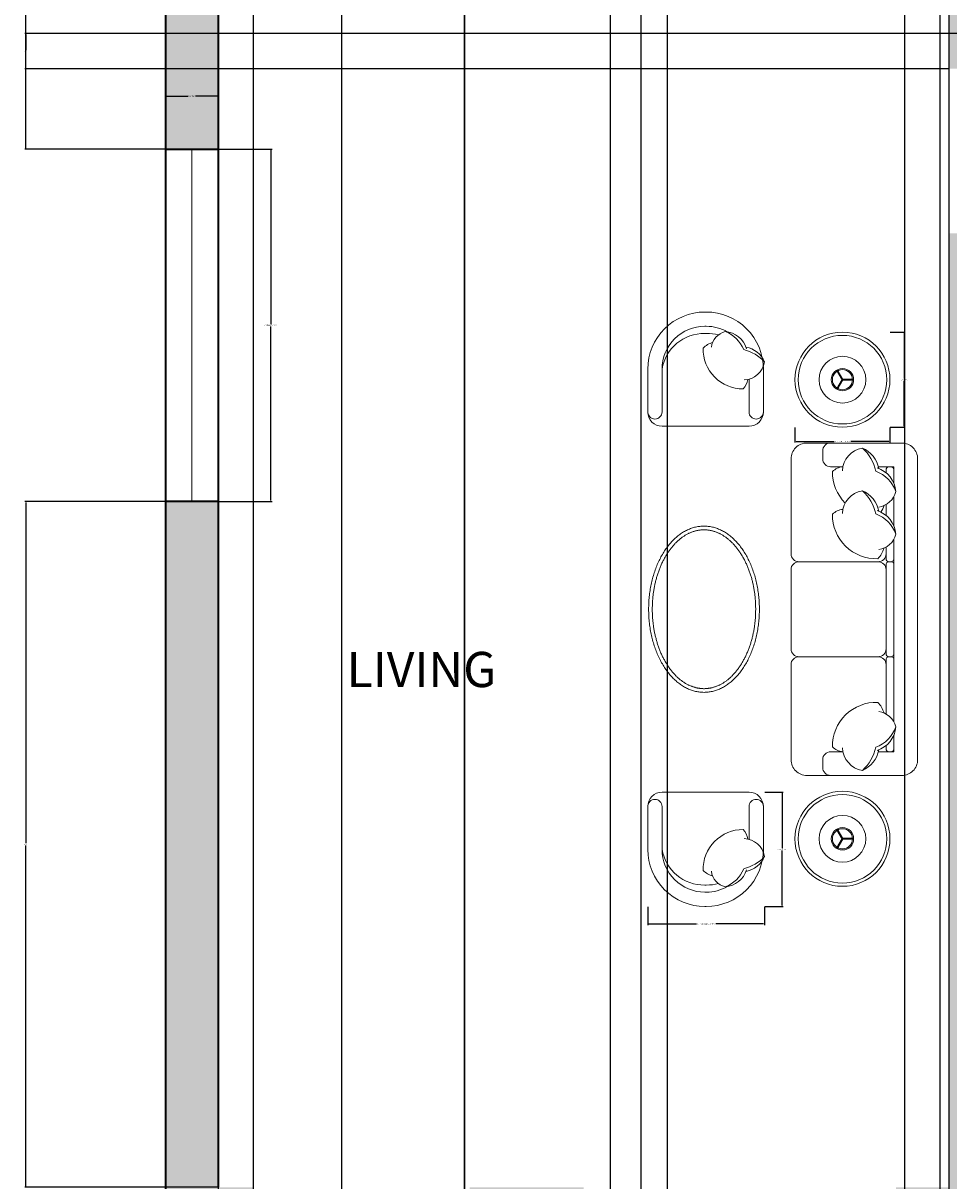
# Model space of a CAD drawing. Units: inches. Extents: x 10 to 332, y -471 to 73.
# Tile 2 of 5: x 10 to 168, y -341 to -144. Entities that reach past the tile are written whole.
import ezdxf

# ---------------------------------------------------------------- set-up
doc = ezdxf.new("R2010")
doc.units = ezdxf.units.IN
doc.header["$MEASUREMENT"] = 0
for name, color, linetype, lineweight in [('A-ANNO-DIMS', 2, 'Continuous', 18), ('A-AREA-IDEN', 7, 'Continuous', 18), ('A-FURN', 9, 'Continuous', 18), ('A-GLAZ', 4, 'Continuous', 18), ('A-WALL', 7, 'Continuous', 35), ('A-WALL-PATT', 8, 'Continuous', 13)]:
    doc.layers.add(name, color=color, linetype=linetype, lineweight=lineweight)
doc.styles.get("Standard").update_dxf_attribs({"font": 'arial.ttf'})
doc.dimstyles.get("Standard").update_dxf_attribs({"dimtxt": 0.18, "dimasz": 0.18, "dimexe": 0.18, "dimexo": 0.0625, "dimgap": 0.09, "dimtad": 0, "dimtih": 1, "dimtoh": 1, "dimdec": 0, "dimzin": 0, "dimdsep": 46, "dimlunit": 3, "dimtxsty": 'Standard', "dimcen": 0.09, "dimadec": 0, "dimazin": 0, "dimtfac": 1, "dimtdec": 0, "dimtofl": 0, "dimtmove": 0, "dimatfit": 3, "dimfxl": 1, "dimtolj": 1, "dimtzin": 0, "dimarcsym": 0})

# ---------------------------------------------------------------- blocks, each defined once
blk = doc.blocks.new('WIN-60')
for p, q in [((0, 9), (60, 9)), ((0, 4.5), (60, 4.5)), ((60, 0), (0, 0))]:
    blk.add_line(p, q)
blk = doc.blocks.new('CHAIR-LOUNGE')
at = {"ltscale": 0.03}
blk.add_lwpolyline([(9.85, 19.45), (2.43, 19.45, 0.414214), (0, 17.02), (0, 9.72, 0.414214), (9.73, 0), (9.85, 0), (9.97, 0, 0.414214), (19.69, 9.72), (19.69, 17.02, 0.414214), (17.26, 19.45), (9.85, 19.45)], format="xyb", dxfattribs=at)
for points in [[(2.43, 9.72), (2.43, 17.02, 0.414214), (1.22, 18.23), (1.22, 18.23, 0.414214), (0, 17.02)], [(17.26, 11.43), (17.26, 17.02, -0.414214), (18.48, 18.23), (18.48, 18.23, -0.414214), (19.69, 17.02)], [(17.02, 11.49, 0.165541), (16.27, 13.09, 0.425989), (9.44, 6.13, 0.121523), (11.06, 5.17, -7.115464)], [(16.41, 11.56, -0.356772), (19.89, 8.5, -0.249542), (16.74, 5.97, 9.61688)], [(2.43, 9.72, 0.372719), (9.73, 3.65), (9.85, 3.65)], [(2.43, 9.72, 0.414214), (9.73, 2.43), (9.85, 2.43)], [(19.89, 8.5, -0.14773), (16.34, 6.41, -0.213343), (13.2, 3.34, -0.178662)], [(16.83, 6.24, -0.306663), (13.2, 3.34, -0.30633), (10.84, 5.99, 0.872847)], [(12.04, 3.91, -0.072384), (9.97, 3.65), (9.85, 3.65)], [(13.59, 3.39, -0.130591), (9.97, 2.43), (9.85, 2.43)]]:
    blk.add_lwpolyline(points, format="xyb")
blk = doc.blocks.new('TABLE-ACCENT-ROUND')
at = {"ltscale": 0.03}
for p, q in [((8.02, 8.05), (7.07, 9.69)), ((8.02, 8.13), (7.07, 6.49)), ((8.16, 8.13), (7.21, 9.78)), ((8.16, 8.05), (7.21, 6.4)), ((8.09, 8.18), (9.99, 8.18)), ((8.09, 8.01), (9.99, 8.01))]:
    blk.add_line(p, q, dxfattribs=at)
for radius in [8.09, 3.98, 1.9, 1.71]:
    blk.add_circle((8.09, 8.09), radius, dxfattribs=at)
blk.add_circle((8.09, 8.09), 7.55)
blk = doc.blocks.new('*D12')
at = {"layer": 'A-ANNO-DIMS', "color": 0, "lineweight": -2, "transparency": 16777216}
for p, q in [((43.43, -165.2), (52.55, -165.2)), ((52.37, -165.38), (52.37, -195.02)), ((52.37, -225.02), (52.37, -195.39)), ((43.43, -225.2), (52.55, -225.2))]:
    blk.add_line(p, q, dxfattribs=at)
at = {"layer": 'A-ANNO-DIMS', "color": 0, "transparency": 16777216}
for points in [[(52.34, -165.38), (52.4, -165.38), (52.37, -165.2)], [(52.34, -225.02), (52.4, -225.02), (52.37, -225.2)]]:
    blk.add_solid(points, dxfattribs=at)
at = {"layer": 'Defpoints', "color": 0, "transparency": 16777216}
for p in [(43.37, -165.2), (43.37, -225.2), (52.37, -225.2)]:
    blk.add_point(p, dxfattribs=at)
at = {"layer": 'A-ANNO-DIMS', "color": 0, "transparency": 16777216, "insert": (52.37, -195.2), "char_height": 0.18, "attachment_point": 5}
blk.add_mtext('\\A1;WINDOW 5\'-0" TYP.', dxfattribs=at)
blk = doc.blocks.new('*D13')
at = {"layer": 'A-ANNO-DIMS', "color": 0, "lineweight": -2, "transparency": 16777216}
for p, q in [((34.37, -165.14), (34.37, -156.02)), ((34.55, -156.2), (38.23, -156.2)), ((43.19, -156.2), (39.51, -156.2)), ((43.37, -165.14), (43.37, -156.02))]:
    blk.add_line(p, q, dxfattribs=at)
at = {"layer": 'A-ANNO-DIMS', "color": 0, "transparency": 16777216}
for points in [[(34.55, -156.17), (34.55, -156.23), (34.37, -156.2)], [(43.19, -156.17), (43.19, -156.23), (43.37, -156.2)]]:
    blk.add_solid(points, dxfattribs=at)
at = {"layer": 'Defpoints', "color": 0, "transparency": 16777216}
for p in [(43.37, -156.2), (34.37, -165.2), (43.37, -165.2)]:
    blk.add_point(p, dxfattribs=at)
at = {"layer": 'A-ANNO-DIMS', "color": 0, "transparency": 16777216, "insert": (38.87, -156.2), "char_height": 0.18, "attachment_point": 5}
blk.add_mtext('\\A1;0\'-9" TYP.', dxfattribs=at)
blk = doc.blocks.new('*D18')
at = {"layer": 'A-ANNO-DIMS', "color": 0, "lineweight": -2, "transparency": 16777216}
for p, q in [((116.57, -294.25), (116.57, -297.35)), ((136.46, -294.25), (136.46, -297.35)), ((116.75, -297.17), (124.89, -297.17)), ((136.28, -297.17), (128.14, -297.17))]:
    blk.add_line(p, q, dxfattribs=at)
at = {"layer": 'A-ANNO-DIMS', "color": 0, "transparency": 16777216}
for points in [[(116.75, -297.14), (116.75, -297.2), (116.57, -297.17)], [(136.28, -297.14), (136.28, -297.2), (136.46, -297.17)]]:
    blk.add_solid(points, dxfattribs=at)
at = {"layer": 'Defpoints', "color": 0, "transparency": 16777216}
for p in [(116.57, -294.18), (136.46, -294.18), (136.46, -297.17)]:
    blk.add_point(p, dxfattribs=at)
at = {"layer": 'A-ANNO-DIMS', "color": 0, "transparency": 16777216, "insert": (126.52, -297.17), "char_height": 0.18, "attachment_point": 5}
blk.add_mtext('\\A1;LOUNGE CHAIR 1\'-8" TYP.', dxfattribs=at)
blk = doc.blocks.new('*D19')
at = {"layer": 'A-ANNO-DIMS', "color": 0, "lineweight": -2, "transparency": 16777216}
for p, q in [((136.53, -274.73), (139.63, -274.73)), ((139.45, -274.91), (139.45, -284.27)), ((139.45, -294), (139.45, -284.64)), ((136.53, -294.18), (139.63, -294.18))]:
    blk.add_line(p, q, dxfattribs=at)
at = {"layer": 'A-ANNO-DIMS', "color": 0, "transparency": 16777216}
for points in [[(139.42, -274.91), (139.48, -274.91), (139.45, -274.73)], [(139.42, -294), (139.48, -294), (139.45, -294.18)]]:
    blk.add_solid(points, dxfattribs=at)
at = {"layer": 'Defpoints', "color": 0, "transparency": 16777216}
for p in [(136.46, -274.73), (139.45, -274.73), (136.46, -294.18)]:
    blk.add_point(p, dxfattribs=at)
at = {"layer": 'A-ANNO-DIMS', "color": 0, "transparency": 16777216, "insert": (139.45, -284.46), "char_height": 0.18, "attachment_point": 5}
blk.add_mtext('\\A1;1\'-7 1/2" TYP.', dxfattribs=at)
blk = doc.blocks.new('*D20')
at = {"layer": 'A-ANNO-DIMS', "color": 0, "lineweight": -2, "transparency": 16777216}
for p, q in [((141.65, -212.61), (141.65, -215.16)), ((157.83, -212.61), (157.83, -215.16)), ((141.83, -214.98), (148.34, -214.98)), ((157.65, -214.98), (151.14, -214.98))]:
    blk.add_line(p, q, dxfattribs=at)
at = {"layer": 'A-ANNO-DIMS', "color": 0, "transparency": 16777216}
for points in [[(141.83, -214.95), (141.83, -215.01), (141.65, -214.98)], [(157.65, -214.95), (157.65, -215.01), (157.83, -214.98)]]:
    blk.add_solid(points, dxfattribs=at)
at = {"layer": 'Defpoints', "color": 0, "transparency": 16777216}
for p in [(141.65, -212.55), (157.83, -212.55), (157.83, -214.98)]:
    blk.add_point(p, dxfattribs=at)
at = {"layer": 'A-ANNO-DIMS', "color": 0, "transparency": 16777216, "insert": (149.74, -214.98), "char_height": 0.18, "attachment_point": 5}
blk.add_mtext('\\A1;SIDE TABLE 1\'-4" TYP.', dxfattribs=at)
blk = doc.blocks.new('*D21')
at = {"layer": 'A-ANNO-DIMS', "color": 0, "lineweight": -2, "transparency": 16777216}
for p, q in [((157.89, -196.37), (160.44, -196.37)), ((160.26, -196.55), (160.26, -204.28)), ((160.26, -212.37), (160.26, -204.64)), ((157.89, -212.55), (160.44, -212.55))]:
    blk.add_line(p, q, dxfattribs=at)
at = {"layer": 'A-ANNO-DIMS', "color": 0, "transparency": 16777216}
for points in [[(160.23, -196.55), (160.29, -196.55), (160.26, -196.37)], [(160.23, -212.37), (160.29, -212.37), (160.26, -212.55)]]:
    blk.add_solid(points, dxfattribs=at)
at = {"layer": 'Defpoints', "color": 0, "transparency": 16777216}
for p in [(157.83, -196.37), (160.26, -196.37), (157.83, -212.55)]:
    blk.add_point(p, dxfattribs=at)
at = {"layer": 'A-ANNO-DIMS', "color": 0, "transparency": 16777216, "insert": (160.26, -204.46), "char_height": 0.18, "attachment_point": 5}
blk.add_mtext('\\A1;1\'-4" TYP.', dxfattribs=at)
blk = doc.blocks.new('*D30')
at = {"layer": 'A-ANNO-DIMS', "color": 0, "lineweight": -2, "transparency": 16777216}
for p, q in [((167.87, -93.08), (167.87, -470.94)), ((43.37, -97.58), (43.37, -470.94)), ((43.55, -470.76), (105.02, -470.76)), ((167.69, -470.76), (106.22, -470.76))]:
    blk.add_line(p, q, dxfattribs=at)
at = {"layer": 'A-ANNO-DIMS', "color": 0, "transparency": 16777216}
for points in [[(43.55, -470.73), (43.55, -470.79), (43.37, -470.76)], [(167.69, -470.73), (167.69, -470.79), (167.87, -470.76)]]:
    blk.add_solid(points, dxfattribs=at)
at = {"layer": 'Defpoints', "color": 0, "transparency": 16777216}
for p in [(167.87, -93.01), (43.37, -97.51), (167.87, -470.76)]:
    blk.add_point(p, dxfattribs=at)
at = {"layer": 'A-ANNO-DIMS', "color": 0, "transparency": 16777216, "insert": (105.62, -470.76), "char_height": 0.18, "attachment_point": 5}
blk.add_mtext('\\A1;10\'-4 1/2"', dxfattribs=at)
blk = doc.blocks.new('*D31')
at = {"layer": 'A-ANNO-DIMS', "color": 0, "lineweight": -2, "transparency": 16777216}
for p, q in [((43.3, -225.2), (10.44, -225.2)), ((10.62, -225.38), (10.62, -283.43)), ((10.62, -341.83), (10.62, -283.79)), ((43.3, -342.01), (10.44, -342.01))]:
    blk.add_line(p, q, dxfattribs=at)
at = {"layer": 'A-ANNO-DIMS', "color": 0, "transparency": 16777216}
for points in [[(10.59, -225.38), (10.65, -225.38), (10.62, -225.2)], [(10.59, -341.83), (10.65, -341.83), (10.62, -342.01)]]:
    blk.add_solid(points, dxfattribs=at)
at = {"layer": 'Defpoints', "color": 0, "transparency": 16777216}
for p in [(43.37, -225.2), (10.62, -342.01), (43.37, -342.01)]:
    blk.add_point(p, dxfattribs=at)
at = {"layer": 'A-ANNO-DIMS', "color": 0, "transparency": 16777216, "insert": (10.62, -283.61), "char_height": 0.18, "attachment_point": 5}
blk.add_mtext('\\A1;9\'-9"', dxfattribs=at)
blk = doc.blocks.new('*D36')
at = {"layer": 'A-ANNO-DIMS', "color": 0, "lineweight": -2, "transparency": 16777216}
for p, q in [((160.37, -346.45), (160.37, 35.92)), ((160.55, 35.74), (163.04, 35.74)), ((166.19, 35.74), (163.7, 35.74)), ((166.37, -346.45), (166.37, 35.92))]:
    blk.add_line(p, q, dxfattribs=at)
at = {"layer": 'A-ANNO-DIMS', "color": 0, "transparency": 16777216}
for points in [[(160.55, 35.77), (160.55, 35.71), (160.37, 35.74)], [(166.19, 35.77), (166.19, 35.71), (166.37, 35.74)]]:
    blk.add_solid(points, dxfattribs=at)
at = {"layer": 'Defpoints', "color": 0, "transparency": 16777216}
for p in [(166.37, 35.74), (160.37, -346.51), (166.37, -346.51)]:
    blk.add_point(p, dxfattribs=at)
at = {"layer": 'A-ANNO-DIMS', "color": 0, "transparency": 16777216, "insert": (163.37, 35.74), "char_height": 0.18, "attachment_point": 5}
blk.add_mtext('\\A1;0\'-6"', dxfattribs=at)
blk = doc.blocks.new('*D40')
at = {"layer": 'A-ANNO-DIMS', "color": 0, "lineweight": -2, "transparency": 16777216}
for p, q in [((43.3, -97.51), (10.44, -97.51)), ((10.62, -97.69), (10.62, -131.18)), ((10.62, -165.02), (10.62, -131.54)), ((43.3, -165.2), (10.44, -165.2))]:
    blk.add_line(p, q, dxfattribs=at)
at = {"layer": 'A-ANNO-DIMS', "color": 0, "transparency": 16777216}
for points in [[(10.59, -97.69), (10.65, -97.69), (10.62, -97.51)], [(10.59, -165.02), (10.65, -165.02), (10.62, -165.2)]]:
    blk.add_solid(points, dxfattribs=at)
at = {"layer": 'Defpoints', "color": 0, "transparency": 16777216}
for p in [(43.37, -97.51), (10.62, -165.2), (43.37, -165.2)]:
    blk.add_point(p, dxfattribs=at)
at = {"layer": 'A-ANNO-DIMS', "color": 0, "transparency": 16777216, "insert": (10.62, -131.36), "char_height": 0.18, "attachment_point": 5}
blk.add_mtext('\\A1;5\'-7 1/2"', dxfattribs=at)
blk = doc.blocks.new('*D46')
at = {"layer": 'A-ANNO-DIMS', "color": 0, "lineweight": -2, "transparency": 16777216}
for p, q in [((43.37, -93.08), (43.37, -470.94)), ((64.36, -93.08), (64.36, -470.94)), ((43.55, -470.76), (53.54, -470.76)), ((64.18, -470.76), (54.18, -470.76))]:
    blk.add_line(p, q, dxfattribs=at)
at = {"layer": 'A-ANNO-DIMS', "color": 0, "transparency": 16777216}
for points in [[(43.55, -470.73), (43.55, -470.79), (43.37, -470.76)], [(64.18, -470.73), (64.18, -470.79), (64.36, -470.76)]]:
    blk.add_solid(points, dxfattribs=at)
at = {"layer": 'Defpoints', "color": 0, "transparency": 16777216}
for p in [(43.37, -93.01), (64.36, -93.01), (64.36, -470.76)]:
    blk.add_point(p, dxfattribs=at)
at = {"layer": 'A-ANNO-DIMS', "color": 0, "transparency": 16777216, "insert": (53.86, -470.76), "char_height": 0.18, "attachment_point": 5}
blk.add_mtext('\\A1;1\'-9"', dxfattribs=at)
blk = doc.blocks.new('*D48')
at = {"layer": 'A-ANNO-DIMS', "color": 0, "lineweight": -2, "transparency": 16777216}
for p, q in [((85.3, -93.08), (85.3, -470.94)), ((110.16, -93.08), (110.16, -470.94)), ((85.48, -470.76), (97.4, -470.76)), ((109.98, -470.76), (98.06, -470.76))]:
    blk.add_line(p, q, dxfattribs=at)
at = {"layer": 'A-ANNO-DIMS', "color": 0, "transparency": 16777216}
for points in [[(85.48, -470.73), (85.48, -470.79), (85.3, -470.76)], [(109.98, -470.73), (109.98, -470.79), (110.16, -470.76)]]:
    blk.add_solid(points, dxfattribs=at)
at = {"layer": 'Defpoints', "color": 0, "transparency": 16777216}
for p in [(85.3, -93.01), (110.16, -93.01), (110.16, -470.76)]:
    blk.add_point(p, dxfattribs=at)
at = {"layer": 'A-ANNO-DIMS', "color": 0, "transparency": 16777216, "insert": (97.73, -470.76), "char_height": 0.18, "attachment_point": 5}
blk.add_mtext('\\A1;2\'-1"', dxfattribs=at)
blk = doc.blocks.new('*D50')
at = {"layer": 'A-ANNO-DIMS', "color": 0, "lineweight": -2, "transparency": 16777216}
for p, q in [((115.37, -93.08), (115.37, -470.94)), ((119.87, -97.58), (119.87, -470.94)), ((115.55, -470.76), (117.08, -470.76)), ((119.69, -470.76), (118.16, -470.76))]:
    blk.add_line(p, q, dxfattribs=at)
at = {"layer": 'A-ANNO-DIMS', "color": 0, "transparency": 16777216}
for points in [[(115.55, -470.73), (115.55, -470.79), (115.37, -470.76)], [(119.69, -470.73), (119.69, -470.79), (119.87, -470.76)]]:
    blk.add_solid(points, dxfattribs=at)
at = {"layer": 'Defpoints', "color": 0, "transparency": 16777216}
for p in [(115.37, -93.01), (119.87, -97.51), (119.87, -470.76)]:
    blk.add_point(p, dxfattribs=at)
at = {"layer": 'A-ANNO-DIMS', "color": 0, "transparency": 16777216, "insert": (117.62, -470.76), "char_height": 0.18, "attachment_point": 5}
blk.add_mtext('\\A1;0\'-4 1/2"', dxfattribs=at)
blk = doc.blocks.new('*D54')
at = {"layer": 'A-ANNO-DIMS', "color": 0, "lineweight": -2, "transparency": 16777216}
for p, q in [((49.37, -418.45), (49.37, 35.92)), ((49.55, 35.74), (67.04, 35.74)), ((85.19, 35.74), (67.7, 35.74)), ((85.37, -418.45), (85.37, 35.92))]:
    blk.add_line(p, q, dxfattribs=at)
at = {"layer": 'A-ANNO-DIMS', "color": 0, "transparency": 16777216}
for points in [[(49.55, 35.77), (49.55, 35.71), (49.37, 35.74)], [(85.19, 35.77), (85.19, 35.71), (85.37, 35.74)]]:
    blk.add_solid(points, dxfattribs=at)
at = {"layer": 'Defpoints', "color": 0, "transparency": 16777216}
for p in [(85.37, 35.74), (49.37, -418.51), (85.37, -418.51)]:
    blk.add_point(p, dxfattribs=at)
at = {"layer": 'A-ANNO-DIMS', "color": 0, "transparency": 16777216, "insert": (67.37, 35.74), "char_height": 0.18, "attachment_point": 5}
blk.add_mtext('\\A1;3\'-0"', dxfattribs=at)
blk = doc.blocks.new('*D58')
at = {"layer": 'A-ANNO-DIMS', "color": 0, "lineweight": -2, "transparency": 16777216}
for p, q in [((172.3, -145.51), (10.44, -145.51)), ((10.62, -145.69), (10.62, -148.33)), ((10.62, -151.33), (10.62, -148.7)), ((167.8, -151.51), (10.44, -151.51))]:
    blk.add_line(p, q, dxfattribs=at)
at = {"layer": 'A-ANNO-DIMS', "color": 0, "transparency": 16777216}
for points in [[(10.59, -145.69), (10.65, -145.69), (10.62, -145.51)], [(10.59, -151.33), (10.65, -151.33), (10.62, -151.51)]]:
    blk.add_solid(points, dxfattribs=at)
at = {"layer": 'Defpoints', "color": 0, "transparency": 16777216}
for p in [(172.37, -145.51), (10.62, -151.51), (167.87, -151.51)]:
    blk.add_point(p, dxfattribs=at)
at = {"layer": 'A-ANNO-DIMS', "color": 0, "transparency": 16777216, "insert": (10.62, -148.51), "char_height": 0.18, "attachment_point": 5}
blk.add_mtext('\\A1;0\'-6"', dxfattribs=at)

msp = doc.modelspace()

# ---------------------------------------------------------------- hatches: boundary and pattern name
at = {"layer": 'A-WALL-PATT'}
h = msp.add_hatch(color=256, dxfattribs=at)
h.dxf.hatch_style = 1
h.paths.add_polyline_path([(132.66, 11.99), (109.37, 11.99), (109.37, 2.99), (115.37, 2.99), (115.37, -93.01), (110.16, -93.01), (110.16, -97.51), (119.87, -97.51), (119.87, -73.51), (167.87, -73.51), (167.87, -107.01), (170.12, -107.01), (172.37, -107.01), (172.37, -63.01), (167.87, -63.01), (167.87, -69.01), (119.87, -69.01), (119.87, 2.99), (132.66, 2.99)])
h.paths.add_polyline_path([(202.37, 11.99), (152.96, 11.99), (152.96, 2.99), (167.87, 2.99), (167.87, -35.01), (170.12, -35.01), (172.37, -35.01), (172.37, 2.99), (202.37, 2.99)])
h.paths.add_polyline_path([(49.37, 11.99), (34.37, 11.99), (34.37, -15.01), (43.37, -15.01), (43.37, 2.99), (49.37, 2.99)])
h.paths.add_polyline_path([(301.37, 11.99), (262.37, 11.99), (262.37, 2.99), (292.37, 2.99), (292.37, -39.01), (301.37, -39.01)])
h.paths.add_polyline_path([(85.3, -93.01), (43.37, -93.01), (43.37, -75.01), (34.37, -75.01), (34.37, -165.2), (43.37, -165.2), (43.37, -97.51), (85.3, -97.51)])
h.paths.add_polyline_path([(43.37, -225.2), (34.37, -225.2), (34.37, -427.51), (49.37, -427.51), (49.37, -418.51), (43.37, -418.51), (43.37, -346.51), (49.4, -346.51), (49.4, -342.01), (43.37, -342.01)])
h.paths.add_polyline_path([(105.62, -342.01), (86.21, -342.01), (86.21, -346.51), (91.37, -346.51), (91.37, -418.51), (85.37, -418.51), (85.37, -427.51), (101.87, -427.51), (101.87, -418.51), (95.87, -418.51), (95.87, -346.51), (105.62, -346.51)])
h.paths.add_polyline_path([(301.37, -312.01), (292.37, -312.01), (292.37, -342.01), (172.37, -342.01), (172.37, -179.51), (170.12, -179.51), (167.87, -179.51), (167.87, -342.01), (158.84, -342.01), (158.84, -346.51), (292.37, -346.51), (292.37, -352.51), (301.37, -352.51)])
h.paths.add_polyline_path([(301.37, -412.51), (292.37, -412.51), (292.37, -418.51), (153.87, -418.51), (153.87, -423.01), (153.87, -427.51), (301.37, -427.51)])
h.paths.add_polyline_path([(301.37, -99.01), (292.37, -99.01), (292.37, -141.01), (172.37, -141.01), (172.37, -135.01), (167.87, -135.01), (167.87, -151.51), (172.37, -151.51), (172.37, -145.51), (292.37, -145.51), (292.37, -165.79), (301.37, -165.79)])

# ---------------------------------------------------------------- linework, layer by layer
at = {"layer": 'A-FURN', "ltscale": 0.03}
msp.add_lwpolyline([(143.68, -271.87, -0.414214), (140.98, -269.18), (140.98, -253, -0.414214), (142.33, -251.65, -0.414214), (140.98, -250.3), (140.98, -236.82, -0.414214), (142.33, -235.47, -0.414214), (140.98, -234.12), (140.98, -217.94, -0.414214), (143.68, -215.25), (159.85, -215.25, -0.414214), (162.55, -217.94), (162.55, -269.18, -0.414214), (159.85, -271.87)], format="xyb", close=True, dxfattribs=at)
at = {"layer": 'A-FURN'}
for points in [[(149.81, -219.29), (147.72, -219.29, -0.414214), (146.37, -217.94), (146.37, -216.59, -0.414214), (147.72, -215.25)], [(149.73, -219.97, -0.356772), (153.13, -216.1, -0.249542), (155.93, -219.6, 9.61688)], [(153.13, -216.1, -0.14773), (155.44, -220.04, -0.213343), (158.84, -223.52, -0.178662)], [(149.81, -219.29, 0.165541), (148.03, -220.12, 0.200231), (150.2, -225.47, 0.121523)], [(155.63, -219.5, -0.306663), (158.84, -223.52, -0.30633), (155.91, -226.15, 0.872847)], [(158.51, -222.13), (158.51, -219.29), (155.86, -219.29, -0.414214)], [(157.16, -220.32), (157.16, -219.83, -0.414214), (157.7, -219.29), (157.97, -219.29, -0.414214), (158.51, -219.83)], [(158.51, -219.83), (158.51, -222.13, -0.414214)], [(149.73, -227.23, -0.356772), (153.13, -223.37, -0.249542), (155.93, -226.87, 9.61688)], [(153.13, -223.37, -0.14773), (155.44, -227.31, -0.213343), (158.84, -230.78, -0.178662)], [(158.51, -224.37), (158.51, -229.39, -0.414214)], [(149.81, -226.55, 0.165541), (148.03, -227.38, 0.425989), (155.75, -234.96, 0.121523), (156.82, -233.16, -7.115464)], [(156.29, -227.03, 0.071865), (156.82, -225.9, -7.115464)], [(157.16, -227.58), (157.16, -225.73, -0.414214)], [(155.63, -226.76, -0.306663), (158.84, -230.78, -0.30633), (155.91, -233.41, 0.872847)], [(158.51, -231.63), (158.51, -234.93, -0.414214), (157.97, -235.47), (157.7, -235.47, -0.414214), (157.16, -234.93), (157.16, -232.99, -0.414214)], [(157.16, -234.12, -0.414214), (155.81, -235.47), (142.33, -235.47, -0.414214)], [(157.16, -236.82, 0.414214), (155.81, -235.47)], [(157.16, -250.3, -0.414214), (155.81, -251.65)], [(157.16, -253, 0.414214), (155.81, -251.65), (142.33, -251.65, 0.414214)], [(158.51, -262.75), (158.51, -252.19, 0.414214), (157.97, -251.65), (157.7, -251.65, 0.414214), (157.16, -252.19), (157.16, -261.39, 0.414214)], [(149.81, -267.83, -0.165541), (148.03, -267, -0.425989), (155.75, -259.42, -0.121523), (156.82, -261.22, 7.115464)], [(155.63, -267.62, 0.306663), (158.84, -263.6, 0.30633), (155.91, -260.97, -0.872847)], [(153.13, -271.01, 0.14773), (155.44, -267.07, 0.213343), (158.84, -263.6, 0.178662)], [(158.51, -267.29), (158.51, -264.99, 0.414214)], [(147.72, -271.87, -0.414214), (146.37, -270.52), (146.37, -269.18, -0.414214), (147.72, -267.83), (149.81, -267.83)], [(149.73, -267.15, 0.356772), (153.13, -271.01, 0.249542), (155.93, -267.51, -9.61688)], [(157.16, -266.8), (157.16, -267.29, 0.414214), (157.7, -267.83), (157.97, -267.83, 0.414214), (158.51, -267.29)]]:
    msp.add_lwpolyline(points, format="xyb", dxfattribs=at)
for points in [[(158.51, -229.39), (158.51, -224.37)], [(158.51, -262.75), (158.51, -231.63)], [(155.86, -267.83), (158.51, -267.83), (158.51, -264.99)]]:
    msp.add_lwpolyline(points, dxfattribs=at)
msp.add_lwpolyline([(158.51, -236.01), (158.51, -251.11, -0.414214), (157.97, -251.65), (157.7, -251.65, -0.414214), (157.16, -251.11), (157.16, -236.01, -0.414214), (157.7, -235.47), (157.97, -235.47, -0.414214)], format="xyb", close=True, dxfattribs=at)
at = {"layer": 'A-FURN', "ltscale": 0.03}
msp.add_polyline3d([(126.15, -257.72, 0), (126.33, -257.71, 0), (126.5, -257.71, 0), (126.68, -257.69, 0), (126.86, -257.68, 0), (127.04, -257.65, 0), (127.22, -257.62, 0), (127.39, -257.59, 0), (127.57, -257.55, 0), (127.75, -257.51, 0), (127.92, -257.46, 0), (128.1, -257.41, 0), (128.27, -257.35, 0), (128.45, -257.29, 0), (128.62, -257.22, 0), (128.79, -257.15, 0), (128.96, -257.07, 0), (129.13, -256.99, 0), (129.3, -256.9, 0), (129.47, -256.81, 0), (129.64, -256.71, 0), (129.8, -256.61, 0), (129.96, -256.51, 0), (130.13, -256.4, 0), (130.29, -256.28, 0), (130.45, -256.16, 0), (130.61, -256.04, 0), (130.76, -255.91, 0), (130.92, -255.77, 0), (131.07, -255.64, 0), (131.22, -255.49, 0), (131.37, -255.35, 0), (131.52, -255.2, 0), (131.67, -255.04, 0), (131.81, -254.88, 0), (131.95, -254.72, 0), (132.09, -254.56, 0), (132.23, -254.38, 0), (132.36, -254.21, 0), (132.5, -254.03, 0), (132.63, -253.85, 0), (132.76, -253.66, 0), (132.88, -253.47, 0), (133.01, -253.28, 0), (133.13, -253.08, 0), (133.25, -252.88, 0), (133.36, -252.68, 0), (133.48, -252.48, 0), (133.59, -252.27, 0), (133.7, -252.05, 0), (133.8, -251.84, 0), (133.91, -251.62, 0), (134.01, -251.4, 0), (134.1, -251.17, 0), (134.2, -250.94, 0), (134.29, -250.71, 0), (134.38, -250.48, 0), (134.47, -250.25, 0), (134.55, -250.01, 0), (134.63, -249.77, 0), (134.71, -249.53, 0), (134.78, -249.28, 0), (134.85, -249.04, 0), (134.92, -248.79, 0), (134.98, -248.54, 0), (135.04, -248.29, 0), (135.1, -248.04, 0), (135.16, -247.78, 0), (135.21, -247.52, 0), (135.26, -247.27, 0), (135.3, -247.01, 0), (135.34, -246.75, 0), (135.38, -246.48, 0), (135.42, -246.22, 0), (135.45, -245.96, 0), (135.48, -245.69, 0), (135.5, -245.43, 0), (135.52, -245.16, 0), (135.54, -244.9, 0), (135.56, -244.63, 0), (135.57, -244.36, 0), (135.58, -244.09, 0), (135.58, -243.83, 0), (135.59, -243.56, 0), (135.58, -243.29, 0), (135.58, -243.02, 0), (135.57, -242.76, 0), (135.56, -242.49, 0), (135.54, -242.22, 0), (135.52, -241.95, 0), (135.5, -241.69, 0), (135.48, -241.42, 0), (135.45, -241.16, 0), (135.42, -240.9, 0), (135.38, -240.63, 0), (135.34, -240.37, 0), (135.3, -240.11, 0), (135.26, -239.85, 0), (135.21, -239.59, 0), (135.16, -239.34, 0), (135.1, -239.08, 0), (135.04, -238.83, 0), (134.98, -238.58, 0), (134.92, -238.33, 0), (134.85, -238.08, 0), (134.78, -237.83, 0), (134.71, -237.59, 0), (134.63, -237.35, 0), (134.55, -237.11, 0), (134.47, -236.87, 0), (134.38, -236.64, 0), (134.29, -236.4, 0), (134.2, -236.17, 0), (134.1, -235.95, 0), (134.01, -235.72, 0), (133.91, -235.5, 0), (133.8, -235.28, 0), (133.7, -235.07, 0), (133.59, -234.85, 0), (133.48, -234.64, 0), (133.36, -234.44, 0), (133.25, -234.23, 0), (133.13, -234.03, 0), (133.01, -233.84, 0), (132.88, -233.64, 0), (132.76, -233.45, 0), (132.63, -233.27, 0), (132.5, -233.09, 0), (132.36, -232.91, 0), (132.23, -232.73, 0), (132.09, -232.56, 0), (131.95, -232.4, 0), (131.81, -232.23, 0), (131.67, -232.07, 0), (131.52, -231.92, 0), (131.37, -231.77, 0), (131.22, -231.62, 0), (131.07, -231.48, 0), (130.92, -231.34, 0), (130.76, -231.21, 0), (130.61, -231.08, 0), (130.45, -230.96, 0), (130.29, -230.84, 0), (130.13, -230.72, 0), (129.96, -230.61, 0), (129.8, -230.51, 0), (129.64, -230.4, 0), (129.47, -230.31, 0), (129.3, -230.22, 0), (129.13, -230.13, 0), (128.96, -230.05, 0), (128.79, -229.97, 0), (128.62, -229.9, 0), (128.45, -229.83, 0), (128.27, -229.77, 0), (128.1, -229.71, 0), (127.92, -229.65, 0), (127.75, -229.61, 0), (127.57, -229.56, 0), (127.39, -229.53, 0), (127.22, -229.49, 0), (127.04, -229.47, 0), (126.86, -229.44, 0), (126.68, -229.42, 0), (126.5, -229.41, 0), (126.33, -229.4, 0), (126.15, -229.4, 0), (125.97, -229.4, 0), (125.79, -229.41, 0), (125.61, -229.42, 0), (125.43, -229.44, 0), (125.26, -229.47, 0), (125.08, -229.49, 0), (124.9, -229.53, 0), (124.72, -229.56, 0), (124.55, -229.61, 0), (124.37, -229.65, 0), (124.2, -229.71, 0), (124.02, -229.77, 0), (123.85, -229.83, 0), (123.68, -229.9, 0), (123.5, -229.97, 0), (123.33, -230.05, 0), (123.16, -230.13, 0), (122.99, -230.22, 0), (122.83, -230.31, 0), (122.66, -230.4, 0), (122.49, -230.51, 0), (122.33, -230.61, 0), (122.17, -230.72, 0), (122.01, -230.84, 0), (121.85, -230.96, 0), (121.69, -231.08, 0), (121.53, -231.21, 0), (121.38, -231.34, 0), (121.22, -231.48, 0), (121.07, -231.62, 0), (120.92, -231.77, 0), (120.77, -231.92, 0), (120.63, -232.07, 0), (120.49, -232.23, 0), (120.34, -232.4, 0), (120.2, -232.56, 0), (120.07, -232.73, 0), (119.93, -232.91, 0), (119.8, -233.09, 0), (119.67, -233.27, 0), (119.54, -233.45, 0), (119.41, -233.64, 0), (119.29, -233.84, 0), (119.17, -234.03, 0), (119.05, -234.23, 0), (118.93, -234.44, 0), (118.82, -234.64, 0), (118.71, -234.85, 0), (118.6, -235.07, 0), (118.49, -235.28, 0), (118.39, -235.5, 0), (118.29, -235.72, 0), (118.19, -235.95, 0), (118.1, -236.17, 0), (118, -236.4, 0), (117.92, -236.64, 0), (117.83, -236.87, 0), (117.75, -237.11, 0), (117.67, -237.35, 0), (117.59, -237.59, 0), (117.52, -237.83, 0), (117.45, -238.08, 0), (117.38, -238.33, 0), (117.31, -238.58, 0), (117.25, -238.83, 0), (117.19, -239.08, 0), (117.14, -239.34, 0), (117.09, -239.59, 0), (117.04, -239.85, 0), (116.99, -240.11, 0), (116.95, -240.37, 0), (116.91, -240.63, 0), (116.88, -240.9, 0), (116.85, -241.16, 0), (116.82, -241.42, 0), (116.79, -241.69, 0), (116.77, -241.95, 0), (116.75, -242.22, 0), (116.74, -242.49, 0), (116.72, -242.76, 0), (116.72, -243.02, 0), (116.71, -243.29, 0), (116.71, -243.56, 0), (116.71, -243.83, 0), (116.72, -244.09, 0), (116.72, -244.36, 0), (116.74, -244.63, 0), (116.75, -244.9, 0), (116.77, -245.16, 0), (116.79, -245.43, 0), (116.82, -245.69, 0), (116.85, -245.96, 0), (116.88, -246.22, 0), (116.91, -246.48, 0), (116.95, -246.75, 0), (116.99, -247.01, 0), (117.04, -247.27, 0), (117.09, -247.52, 0), (117.14, -247.78, 0), (117.19, -248.04, 0), (117.25, -248.29, 0), (117.31, -248.54, 0), (117.38, -248.79, 0), (117.45, -249.04, 0), (117.52, -249.28, 0), (117.59, -249.53, 0), (117.67, -249.77, 0), (117.75, -250.01, 0), (117.83, -250.25, 0), (117.92, -250.48, 0), (118, -250.71, 0), (118.1, -250.94, 0), (118.19, -251.17, 0), (118.29, -251.4, 0), (118.39, -251.62, 0), (118.49, -251.84, 0), (118.6, -252.05, 0), (118.71, -252.27, 0), (118.82, -252.48, 0), (118.93, -252.68, 0), (119.05, -252.88, 0), (119.17, -253.08, 0), (119.29, -253.28, 0), (119.41, -253.47, 0), (119.54, -253.66, 0), (119.67, -253.85, 0), (119.8, -254.03, 0), (119.93, -254.21, 0), (120.07, -254.38, 0), (120.2, -254.56, 0), (120.34, -254.72, 0), (120.49, -254.88, 0), (120.63, -255.04, 0), (120.77, -255.2, 0), (120.92, -255.35, 0), (121.07, -255.49, 0), (121.22, -255.64, 0), (121.38, -255.77, 0), (121.53, -255.91, 0), (121.69, -256.04, 0), (121.85, -256.16, 0), (122.01, -256.28, 0), (122.17, -256.4, 0), (122.33, -256.51, 0), (122.49, -256.61, 0), (122.66, -256.71, 0), (122.83, -256.81, 0), (122.99, -256.9, 0), (123.16, -256.99, 0), (123.33, -257.07, 0), (123.5, -257.15, 0), (123.68, -257.22, 0), (123.85, -257.29, 0), (124.02, -257.35, 0), (124.2, -257.41, 0), (124.37, -257.46, 0), (124.55, -257.51, 0), (124.72, -257.55, 0), (124.9, -257.59, 0), (125.08, -257.62, 0), (125.26, -257.65, 0), (125.43, -257.68, 0), (125.61, -257.69, 0), (125.79, -257.71, 0), (125.97, -257.71, 0), (126.15, -257.72, 0)], dxfattribs=at)
at = {"layer": 'A-FURN'}
msp.add_polyline3d([(126.15, -257.09, 0), (126.24, -257.09, 0), (126.34, -257.08, 0), (126.44, -257.08, 0), (126.54, -257.07, 0), (126.63, -257.07, 0), (126.73, -257.06, 0), (126.83, -257.05, 0), (126.93, -257.03, 0), (127.03, -257.02, 0), (127.13, -257, 0), (127.23, -256.98, 0), (127.33, -256.96, 0), (127.43, -256.94, 0), (127.53, -256.92, 0), (127.64, -256.89, 0), (127.74, -256.86, 0), (127.84, -256.83, 0), (127.94, -256.8, 0), (128.04, -256.77, 0), (128.15, -256.73, 0), (128.25, -256.69, 0), (128.35, -256.65, 0), (128.46, -256.61, 0), (128.56, -256.56, 0), (128.66, -256.52, 0), (128.77, -256.47, 0), (128.87, -256.42, 0), (128.97, -256.36, 0), (129.08, -256.31, 0), (129.18, -256.25, 0), (129.28, -256.19, 0), (129.39, -256.13, 0), (129.49, -256.07, 0), (129.59, -256, 0), (129.69, -255.93, 0), (129.8, -255.86, 0), (129.9, -255.79, 0), (130, -255.71, 0), (130.1, -255.64, 0), (130.2, -255.56, 0), (130.3, -255.47, 0), (130.4, -255.39, 0), (130.5, -255.3, 0), (130.6, -255.22, 0), (130.7, -255.13, 0), (130.79, -255.03, 0), (130.89, -254.94, 0), (130.99, -254.84, 0), (131.08, -254.74, 0), (131.18, -254.64, 0), (131.27, -254.53, 0), (131.37, -254.43, 0), (131.46, -254.32, 0), (131.55, -254.21, 0), (131.64, -254.1, 0), (131.73, -253.98, 0), (131.82, -253.87, 0), (131.91, -253.75, 0), (132, -253.63, 0), (132.09, -253.51, 0), (132.17, -253.39, 0), (132.26, -253.26, 0), (132.34, -253.13, 0), (132.43, -253.01, 0), (132.51, -252.88, 0), (132.59, -252.74, 0), (132.67, -252.61, 0), (132.75, -252.48, 0), (132.83, -252.34, 0), (132.9, -252.2, 0), (132.98, -252.06, 0), (133.05, -251.92, 0), (133.13, -251.78, 0), (133.2, -251.64, 0), (133.27, -251.49, 0), (133.34, -251.34, 0), (133.4, -251.2, 0), (133.47, -251.05, 0), (133.54, -250.9, 0), (133.6, -250.75, 0), (133.66, -250.6, 0), (133.72, -250.44, 0), (133.78, -250.29, 0), (133.84, -250.13, 0), (133.89, -249.98, 0), (133.95, -249.82, 0), (134, -249.66, 0), (134.05, -249.51, 0), (134.1, -249.35, 0), (134.15, -249.19, 0), (134.2, -249.03, 0), (134.24, -248.88, 0), (134.29, -248.72, 0), (134.33, -248.56, 0), (134.37, -248.4, 0), (134.41, -248.24, 0), (134.45, -248.08, 0), (134.49, -247.92, 0), (134.52, -247.76, 0), (134.55, -247.6, 0), (134.59, -247.44, 0), (134.62, -247.28, 0), (134.65, -247.11, 0), (134.68, -246.95, 0), (134.7, -246.79, 0), (134.73, -246.63, 0), (134.75, -246.46, 0), (134.77, -246.3, 0), (134.8, -246.14, 0), (134.82, -245.98, 0), (134.83, -245.81, 0), (134.85, -245.65, 0), (134.87, -245.49, 0), (134.88, -245.32, 0), (134.9, -245.16, 0), (134.91, -245, 0), (134.92, -244.83, 0), (134.93, -244.67, 0), (134.94, -244.5, 0), (134.94, -244.34, 0), (134.95, -244.17, 0), (134.95, -244.01, 0), (134.95, -243.85, 0), (134.96, -243.68, 0), (134.96, -243.52, 0), (134.96, -243.35, 0), (134.95, -243.19, 0), (134.95, -243.03, 0), (134.94, -242.86, 0), (134.94, -242.7, 0), (134.93, -242.53, 0), (134.92, -242.37, 0), (134.91, -242.2, 0), (134.9, -242.04, 0), (134.89, -241.88, 0), (134.88, -241.71, 0), (134.86, -241.55, 0), (134.84, -241.39, 0), (134.83, -241.22, 0), (134.81, -241.06, 0), (134.79, -240.9, 0), (134.76, -240.73, 0), (134.74, -240.57, 0), (134.72, -240.41, 0), (134.69, -240.25, 0), (134.66, -240.09, 0), (134.63, -239.92, 0), (134.6, -239.76, 0), (134.57, -239.6, 0), (134.54, -239.44, 0), (134.5, -239.28, 0), (134.47, -239.12, 0), (134.43, -238.96, 0), (134.39, -238.8, 0), (134.35, -238.64, 0), (134.31, -238.48, 0), (134.27, -238.32, 0), (134.22, -238.16, 0), (134.17, -238, 0), (134.13, -237.85, 0), (134.08, -237.69, 0), (134.03, -237.53, 0), (133.98, -237.38, 0), (133.92, -237.22, 0), (133.87, -237.06, 0), (133.81, -236.91, 0), (133.75, -236.75, 0), (133.69, -236.6, 0), (133.63, -236.45, 0), (133.57, -236.29, 0), (133.5, -236.14, 0), (133.44, -235.99, 0), (133.37, -235.85, 0), (133.3, -235.7, 0), (133.23, -235.55, 0), (133.16, -235.41, 0), (133.09, -235.27, 0), (133.02, -235.13, 0), (132.94, -234.99, 0), (132.87, -234.85, 0), (132.79, -234.71, 0), (132.71, -234.57, 0), (132.63, -234.44, 0), (132.55, -234.31, 0), (132.47, -234.18, 0), (132.39, -234.05, 0), (132.3, -233.92, 0), (132.22, -233.79, 0), (132.13, -233.67, 0), (132.04, -233.55, 0), (131.96, -233.43, 0), (131.87, -233.31, 0), (131.78, -233.19, 0), (131.69, -233.08, 0), (131.6, -232.96, 0), (131.51, -232.85, 0), (131.41, -232.74, 0), (131.32, -232.64, 0), (131.23, -232.53, 0), (131.13, -232.43, 0), (131.04, -232.33, 0), (130.94, -232.23, 0), (130.84, -232.13, 0), (130.74, -232.04, 0), (130.65, -231.95, 0), (130.55, -231.86, 0), (130.45, -231.77, 0), (130.35, -231.69, 0), (130.25, -231.6, 0), (130.15, -231.52, 0), (130.05, -231.44, 0), (129.95, -231.37, 0), (129.85, -231.29, 0), (129.74, -231.22, 0), (129.64, -231.15, 0), (129.54, -231.09, 0), (129.44, -231.02, 0), (129.33, -230.96, 0), (129.23, -230.9, 0), (129.13, -230.84, 0), (129.02, -230.78, 0), (128.92, -230.73, 0), (128.82, -230.68, 0), (128.71, -230.63, 0), (128.61, -230.58, 0), (128.51, -230.53, 0), (128.4, -230.49, 0), (128.3, -230.45, 0), (128.2, -230.41, 0), (128.1, -230.37, 0), (127.99, -230.34, 0), (127.89, -230.3, 0), (127.79, -230.27, 0), (127.69, -230.24, 0), (127.59, -230.21, 0), (127.48, -230.19, 0), (127.38, -230.17, 0), (127.28, -230.15, 0), (127.18, -230.13, 0), (127.08, -230.11, 0), (126.98, -230.09, 0), (126.88, -230.08, 0), (126.78, -230.07, 0), (126.68, -230.06, 0), (126.59, -230.05, 0), (126.49, -230.04, 0), (126.39, -230.04, 0), (126.29, -230.03, 0), (126.2, -230.03, 0), (126.1, -230.03, 0), (126, -230.03, 0), (125.91, -230.04, 0), (125.81, -230.04, 0), (125.71, -230.05, 0), (125.61, -230.06, 0), (125.51, -230.07, 0), (125.41, -230.08, 0), (125.31, -230.09, 0), (125.21, -230.11, 0), (125.11, -230.13, 0), (125.01, -230.15, 0), (124.91, -230.17, 0), (124.81, -230.19, 0), (124.71, -230.21, 0), (124.61, -230.24, 0), (124.51, -230.27, 0), (124.4, -230.3, 0), (124.3, -230.34, 0), (124.2, -230.37, 0), (124.1, -230.41, 0), (123.99, -230.45, 0), (123.89, -230.49, 0), (123.79, -230.53, 0), (123.68, -230.58, 0), (123.58, -230.63, 0), (123.48, -230.68, 0), (123.37, -230.73, 0), (123.27, -230.78, 0), (123.17, -230.84, 0), (123.06, -230.9, 0), (122.96, -230.96, 0), (122.86, -231.02, 0), (122.76, -231.09, 0), (122.65, -231.15, 0), (122.55, -231.22, 0), (122.45, -231.29, 0), (122.35, -231.37, 0), (122.25, -231.44, 0), (122.15, -231.52, 0), (122.05, -231.6, 0), (121.95, -231.69, 0), (121.85, -231.77, 0), (121.75, -231.86, 0), (121.65, -231.95, 0), (121.55, -232.04, 0), (121.45, -232.13, 0), (121.36, -232.23, 0), (121.26, -232.33, 0), (121.16, -232.43, 0), (121.07, -232.53, 0), (120.98, -232.64, 0), (120.88, -232.74, 0), (120.79, -232.85, 0), (120.7, -232.96, 0), (120.61, -233.08, 0), (120.52, -233.19, 0), (120.43, -233.31, 0), (120.34, -233.43, 0), (120.25, -233.55, 0), (120.16, -233.67, 0), (120.08, -233.79, 0), (119.99, -233.92, 0), (119.91, -234.05, 0), (119.83, -234.18, 0), (119.75, -234.31, 0), (119.66, -234.44, 0), (119.59, -234.57, 0), (119.51, -234.71, 0), (119.43, -234.85, 0), (119.35, -234.99, 0), (119.28, -235.13, 0), (119.21, -235.27, 0), (119.13, -235.41, 0), (119.06, -235.55, 0), (118.99, -235.7, 0), (118.92, -235.85, 0), (118.86, -235.99, 0), (118.79, -236.14, 0), (118.73, -236.29, 0), (118.66, -236.45, 0), (118.6, -236.6, 0), (118.54, -236.75, 0), (118.49, -236.91, 0), (118.43, -237.06, 0), (118.37, -237.22, 0), (118.32, -237.38, 0), (118.27, -237.53, 0), (118.22, -237.69, 0), (118.17, -237.85, 0), (118.12, -238, 0), (118.07, -238.16, 0), (118.03, -238.32, 0), (117.99, -238.48, 0), (117.94, -238.64, 0), (117.9, -238.8, 0), (117.87, -238.96, 0), (117.83, -239.12, 0), (117.79, -239.28, 0), (117.76, -239.44, 0), (117.72, -239.6, 0), (117.69, -239.76, 0), (117.66, -239.92, 0), (117.63, -240.09, 0), (117.61, -240.25, 0), (117.58, -240.41, 0), (117.56, -240.57, 0), (117.53, -240.73, 0), (117.51, -240.9, 0), (117.49, -241.06, 0), (117.47, -241.22, 0), (117.45, -241.39, 0), (117.44, -241.55, 0), (117.42, -241.71, 0), (117.41, -241.88, 0), (117.39, -242.04, 0), (117.38, -242.2, 0), (117.37, -242.37, 0), (117.36, -242.53, 0), (117.36, -242.7, 0), (117.35, -242.86, 0), (117.35, -243.03, 0), (117.34, -243.19, 0), (117.34, -243.35, 0), (117.34, -243.52, 0), (117.34, -243.68, 0), (117.34, -243.85, 0), (117.34, -244.01, 0), (117.35, -244.17, 0), (117.35, -244.34, 0), (117.36, -244.5, 0), (117.37, -244.67, 0), (117.38, -244.83, 0), (117.39, -245, 0), (117.4, -245.16, 0), (117.41, -245.32, 0), (117.43, -245.49, 0), (117.44, -245.65, 0), (117.46, -245.81, 0), (117.48, -245.98, 0), (117.5, -246.14, 0), (117.52, -246.3, 0), (117.54, -246.46, 0), (117.57, -246.63, 0), (117.59, -246.79, 0), (117.62, -246.95, 0), (117.65, -247.11, 0), (117.68, -247.28, 0), (117.71, -247.44, 0), (117.74, -247.6, 0), (117.77, -247.76, 0), (117.81, -247.92, 0), (117.85, -248.08, 0), (117.88, -248.24, 0), (117.92, -248.4, 0), (117.97, -248.56, 0), (118.01, -248.72, 0), (118.05, -248.88, 0), (118.1, -249.03, 0), (118.14, -249.19, 0), (118.19, -249.35, 0), (118.24, -249.51, 0), (118.29, -249.66, 0), (118.35, -249.82, 0), (118.4, -249.98, 0), (118.46, -250.13, 0), (118.51, -250.29, 0), (118.57, -250.44, 0), (118.63, -250.6, 0), (118.7, -250.75, 0), (118.76, -250.9, 0), (118.82, -251.05, 0), (118.89, -251.2, 0), (118.96, -251.34, 0), (119.03, -251.49, 0), (119.1, -251.64, 0), (119.17, -251.78, 0), (119.24, -251.92, 0), (119.32, -252.06, 0), (119.39, -252.2, 0), (119.47, -252.34, 0), (119.55, -252.48, 0), (119.62, -252.61, 0), (119.7, -252.74, 0), (119.79, -252.88, 0), (119.87, -253.01, 0), (119.95, -253.13, 0), (120.04, -253.26, 0), (120.12, -253.39, 0), (120.21, -253.51, 0), (120.29, -253.63, 0), (120.38, -253.75, 0), (120.47, -253.87, 0), (120.56, -253.98, 0), (120.65, -254.1, 0), (120.74, -254.21, 0), (120.84, -254.32, 0), (120.93, -254.43, 0), (121.02, -254.53, 0), (121.12, -254.64, 0), (121.21, -254.74, 0), (121.31, -254.84, 0), (121.4, -254.94, 0), (121.5, -255.03, 0), (121.6, -255.13, 0), (121.7, -255.22, 0), (121.8, -255.3, 0), (121.9, -255.39, 0), (122, -255.47, 0), (122.1, -255.56, 0), (122.2, -255.64, 0), (122.3, -255.71, 0), (122.4, -255.79, 0), (122.5, -255.86, 0), (122.6, -255.93, 0), (122.7, -256, 0), (122.81, -256.07, 0), (122.91, -256.13, 0), (123.01, -256.19, 0), (123.12, -256.25, 0), (123.22, -256.31, 0), (123.32, -256.36, 0), (123.43, -256.42, 0), (123.53, -256.47, 0), (123.63, -256.52, 0), (123.74, -256.56, 0), (123.84, -256.61, 0), (123.94, -256.65, 0), (124.05, -256.69, 0), (124.15, -256.73, 0), (124.25, -256.77, 0), (124.35, -256.8, 0), (124.46, -256.83, 0), (124.56, -256.86, 0), (124.66, -256.89, 0), (124.76, -256.92, 0), (124.86, -256.94, 0), (124.96, -256.96, 0), (125.06, -256.98, 0), (125.16, -257, 0), (125.26, -257.02, 0), (125.36, -257.03, 0), (125.46, -257.05, 0), (125.56, -257.06, 0), (125.66, -257.07, 0), (125.76, -257.07, 0), (125.86, -257.08, 0), (125.95, -257.08, 0), (126.05, -257.09, 0), (126.15, -257.09, 0)], dxfattribs=at)
at = {"layer": 'A-WALL'}
for p, q in [((34.37, 11.99), (34.37, -427.51)), ((43.37, -97.51), (43.37, -342.01)), ((34.37, -165.2), (43.37, -165.2)), ((43.37, -225.2), (34.37, -225.2))]:
    msp.add_line(p, q, dxfattribs=at)

# ---------------------------------------------------------------- block references
at = {"layer": 'A-FURN', "extrusion": (0, 0, -1), "zscale": -1, "rotation": 180.0000106977531}
msp.add_blockref('CHAIR-LOUNGE', (-116.57, -192.94), dxfattribs=at)
at = {"layer": 'A-FURN'}
for name, p in [('TABLE-ACCENT-ROUND', (141.65, -212.55)), ('CHAIR-LOUNGE', (116.57, -294.18)), ('TABLE-ACCENT-ROUND', (141.65, -290.75))]:
    msp.add_blockref(name, p, dxfattribs=at)
at = {"layer": 'A-GLAZ', "rotation": 270}
msp.add_blockref('WIN-60', (34.37, -165.2), dxfattribs=at)

# ---------------------------------------------------------------- texts
at = {"layer": 'A-AREA-IDEN', "insert": (65.25, -250.82), "char_height": 6, "attachment_point": 1}
msp.add_mtext('LIVING', dxfattribs=at)

# ---------------------------------------------------------------- dimensions: what is measured, and where the dimension line sits
at = {"layer": 'A-ANNO-DIMS'}
for base, p1, p2, picture, middle in [((85.37, 35.74), (49.37, -418.51), (85.37, -418.51), '*D54', (67.37, 35.74)), ((166.37, 35.74), (160.37, -346.51), (166.37, -346.51), '*D36', (163.37, 35.74)), ((167.87, -470.76), (43.37, -97.51), (167.87, -93.01), '*D30', (105.62, -470.76)), ((64.36, -470.76), (43.37, -93.01), (64.36, -93.01), '*D46', (53.86, -470.76)), ((110.16, -470.76), (85.3, -93.01), (110.16, -93.01), '*D48', (97.73, -470.76)), ((119.87, -470.76), (115.37, -93.01), (119.87, -97.51), '*D50', (117.62, -470.76))]:
    dim = msp.add_linear_dim(base=base, p1=p1, p2=p2, dimstyle='Standard', override={"dimdec": 1, "dimlfac": 1, "dimrnd": 0, "dimzin": 1, "dimdsep": 46, "dimlunit": 4, "dimfrac": 2}, dxfattribs=at)
    dim.commit()
    dim.dimension.update_dxf_attribs({"geometry": picture, "text_midpoint": middle})
for base, p1, p2, picture, middle in [((10.62, -165.2), (43.37, -97.51), (43.37, -165.2), '*D40', (10.62, -131.36)), ((10.62, -151.51), (172.37, -145.51), (167.87, -151.51), '*D58', (10.62, -148.51)), ((10.62, -342.01), (43.37, -225.2), (43.37, -342.01), '*D31', (10.62, -283.61))]:
    dim = msp.add_linear_dim(base=base, p1=p1, p2=p2, angle=90, dimstyle='Standard', override={"dimdec": 1, "dimlfac": 1, "dimrnd": 0, "dimzin": 1, "dimdsep": 46, "dimlunit": 4, "dimfrac": 2}, dxfattribs=at)
    dim.commit()
    dim.dimension.update_dxf_attribs({"geometry": picture, "text_midpoint": middle})
for base, p1, p2, text, picture, middle in [((43.37, -156.2), (34.37, -165.2), (43.37, -165.2), '<> TYP.', '*D13', (38.87, -156.2)), ((157.83, -214.98), (141.65, -212.55), (157.83, -212.55), 'SIDE TABLE <> TYP.', '*D20', (149.74, -214.98)), ((136.46, -297.17), (116.57, -294.18), (136.46, -294.18), 'LOUNGE CHAIR <> TYP.', '*D18', (126.52, -297.17))]:
    dim = msp.add_linear_dim(base=base, p1=p1, p2=p2, text=text, dimstyle='Standard', override={"dimdec": 1, "dimlfac": 1, "dimrnd": 0, "dimzin": 1, "dimdsep": 46, "dimlunit": 4, "dimfrac": 2}, dxfattribs=at)
    dim.commit()
    dim.dimension.update_dxf_attribs({"geometry": picture, "text_midpoint": middle})
for base, p1, p2, angle, text, picture, middle in [((52.37, -225.2), (43.37, -165.2), (43.37, -225.2), 270, 'WINDOW <> TYP.', '*D12', (52.37, -195.2)), ((160.26, -196.37), (157.83, -212.55), (157.83, -196.37), 90, '<> TYP.', '*D21', (160.26, -204.46)), ((139.4468, -274.7328), (136.4629, -294.1833), (136.4629, -274.7328), 90, '<> TYP.', '*D19', (139.4468, -284.4581))]:
    dim = msp.add_linear_dim(base=base, p1=p1, p2=p2, angle=angle, text=text, dimstyle='Standard', override={"dimdec": 1, "dimlfac": 1, "dimrnd": 0, "dimzin": 1, "dimdsep": 46, "dimlunit": 4, "dimfrac": 2}, dxfattribs=at)
    dim.commit()
    dim.dimension.update_dxf_attribs({"geometry": picture, "text_midpoint": middle})

doc.saveas('drawing.dxf')
